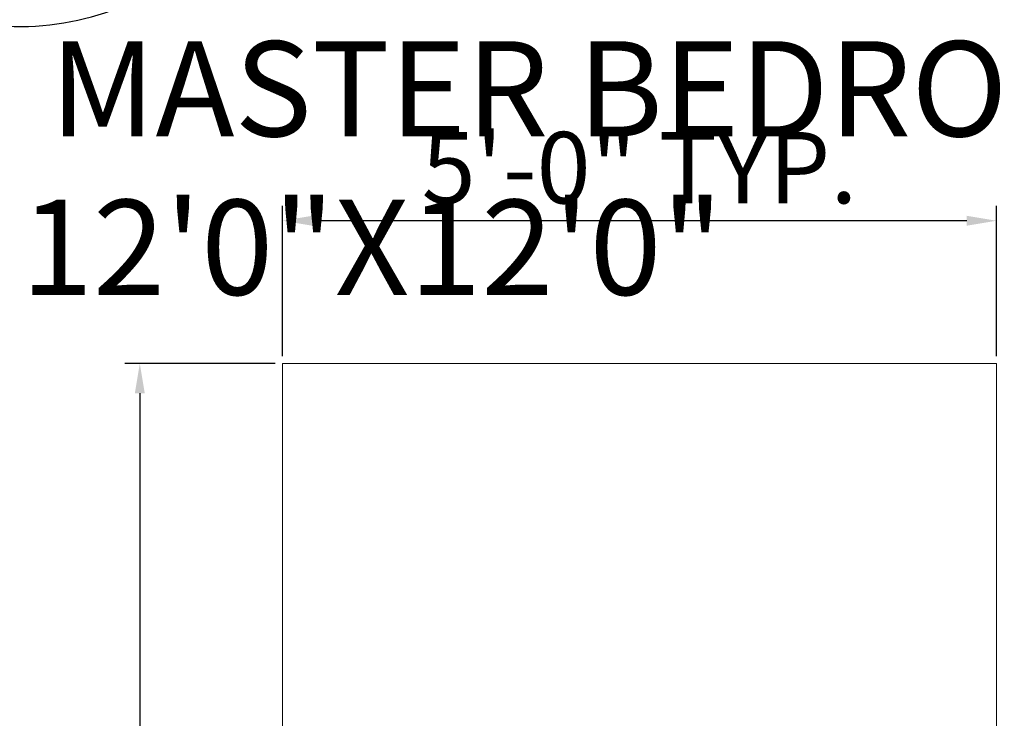
# Model space of a CAD drawing. Units: inches. Extents: x 459864 to 460310, y 324185 to 324787.
# Tile 71 of 112: x 460127 to 460210, y 324341 to 324400. Entities that reach past the tile are written whole.
import ezdxf

# ---------------------------------------------------------------- set-up
doc = ezdxf.new("R2010")
doc.units = ezdxf.units.IN
for name, color, linetype, lineweight in [('A-ANNO-DIMS', 2, 'Continuous', 18), ('A-AREA-IDEN', 7, 'Continuous', 25), ('A-DOOR', 3, 'Continuous', 25), ('A-FURN', 8, 'Continuous', 18)]:
    doc.layers.add(name, color=color, linetype=linetype, lineweight=lineweight)
doc.styles.get("Standard").update_dxf_attribs({"font": 'arial.ttf'})
doc.dimstyles.new('ISO-25', dxfattribs={"dimtxt": 6, "dimasz": 2.5, "dimexe": 1.25, "dimexo": 0.625, "dimtad": 1, "dimdec": 1, "dimlunit": 3, "dimtxsty": 'Standard', "dimcen": 2.5, "dimadec": 0, "dimazin": 0, "dimtfac": 1, "dimtdec": 1, "dimtmove": 0, "dimatfit": 3, "dimfxl": 1, "dimarcsym": 0})

# ---------------------------------------------------------------- blocks, each defined once
blk = doc.blocks.new('Bed - Queen')
for p, q in [((0, -80.00003), (0, 0)), ((0, 0), (59.99999, 0)), ((59.99999, 0), (59.99999, -80.00003)), ((7.99999, -1.2), (28.79998, -1.2)), ((7.99999, -14.4), (7.99999, -1.2)), ((28.79998, -1.2), (28.79998, -14.4)), ((31.19999, -1.2), (51.99999, -1.2)), ((31.19999, -14.4), (31.19999, -1.2)), ((51.99999, -1.2), (51.99999, -16.4)), ((0, -14.4), (44.8, -14.4)), ((59.99999, -29.6), (44.8, -14.4)), ((44.8, -14.4), (44.8, -29.6)), ((51.99999, -16.4), (46.79936, -16.4)), ((44.8, -16.8), (0, -16.8)), ((44.8, -29.6), (59.99999, -29.6)), ((59.99999, -80.00003), (0, -80.00003))]:
    blk.add_line(p, q)
blk = doc.blocks.new('*D28')
at = {"layer": 'A-ANNO-DIMS', "color": 0, "lineweight": -2, "transparency": 16777216}
for p, q in [((460148.65, 324370.7), (460136.025, 324370.7)), ((460137.275, 324368.2), (460137.275, 324293.2)), ((460148.65, 324290.7), (460136.025, 324290.7)), ((460137.275, 324290.7), (460137.275, 324198.69))]:
    blk.add_line(p, q, dxfattribs=at)
at = {"layer": 'A-ANNO-DIMS', "color": 0, "transparency": 16777216}
for points in [[(460136.858, 324368.2), (460137.692, 324368.2), (460137.275, 324370.7)], [(460136.858, 324293.2), (460137.692, 324293.2), (460137.275, 324290.7)]]:
    blk.add_solid(points, dxfattribs=at)
at = {"layer": 'Defpoints', "color": 0, "transparency": 16777216}
for p in [(460149.275, 324370.7), (460137.275, 324290.7), (460149.275, 324290.7)]:
    blk.add_point(p, dxfattribs=at)
at = {"layer": 'A-ANNO-DIMS', "color": 0, "transparency": 16777216, "insert": (460133.363, 324243.445), "char_height": 6, "attachment_point": 5, "rotation": 90}
blk.add_mtext('QUEEN BED 6\'-8" TYP.', dxfattribs=at)
blk = doc.blocks.new('*D29')
at = {"layer": 'A-ANNO-DIMS', "color": 0, "lineweight": -2, "transparency": 16777216}
for p, q in [((460149.275, 324371.325), (460149.275, 324383.95)), ((460209.275, 324371.325), (460209.275, 324383.95)), ((460206.775, 324382.7), (460151.775, 324382.7))]:
    blk.add_line(p, q, dxfattribs=at)
at = {"layer": 'A-ANNO-DIMS', "color": 0, "transparency": 16777216}
for points in [[(460151.775, 324383.117), (460151.775, 324382.284), (460149.275, 324382.7)], [(460206.775, 324383.117), (460206.775, 324382.284), (460209.275, 324382.7)]]:
    blk.add_solid(points, dxfattribs=at)
at = {"layer": 'Defpoints', "color": 0, "transparency": 16777216}
for p in [(460149.275, 324382.7), (460149.275, 324370.7), (460209.275, 324370.7)]:
    blk.add_point(p, dxfattribs=at)
at = {"layer": 'A-ANNO-DIMS', "color": 0, "transparency": 16777216, "insert": (460179.275, 324386.389), "char_height": 6, "attachment_point": 5}
blk.add_mtext('5\'-0" TYP.', dxfattribs=at)

msp = doc.modelspace()

# ---------------------------------------------------------------- linework, layer by layer
at = {"layer": 'A-DOOR'}
msp.add_arc((460127.115, 324422.05), 23.022, 267.51045, 2.48955, dxfattribs=at)

# ---------------------------------------------------------------- block references
at = {"layer": 'A-FURN', "rotation": 180}
msp.add_blockref('Bed - Queen', (460209.275, 324290.7), dxfattribs=at)

# ---------------------------------------------------------------- texts
at = {"layer": 'A-AREA-IDEN', "insert": (460127.286, 324397.798), "char_height": 8, "attachment_point": 1}
msp.add_mtext(' MASTER BEDROOM\\P12\'0"X12\'0"', dxfattribs=at)

# ---------------------------------------------------------------- dimensions: what is measured, and where the dimension line sits
at = {"layer": 'A-ANNO-DIMS'}
for base, p1, p2, angle, text, picture, middle in [((460149.275, 324382.7), (460209.275, 324370.7), (460149.275, 324370.7), 180, '<> TYP.', '*D29', (460179.275, 324386.389)), ((460137.275, 324290.7), (460149.275, 324370.7), (460149.275, 324290.7), 270, 'QUEEN BED <> TYP.', '*D28', (460133.363, 324243.445))]:
    dim = msp.add_linear_dim(base=base, p1=p1, p2=p2, angle=angle, text=text, dimstyle='ISO-25', override={"dimdec": 1, "dimlfac": 1, "dimrnd": 0, "dimzin": 1, "dimdsep": 46, "dimlunit": 4, "dimfrac": 2}, dxfattribs=at)
    dim.commit()
    dim.dimension.update_dxf_attribs({"geometry": picture, "text_midpoint": middle})

doc.saveas('drawing.dxf')
